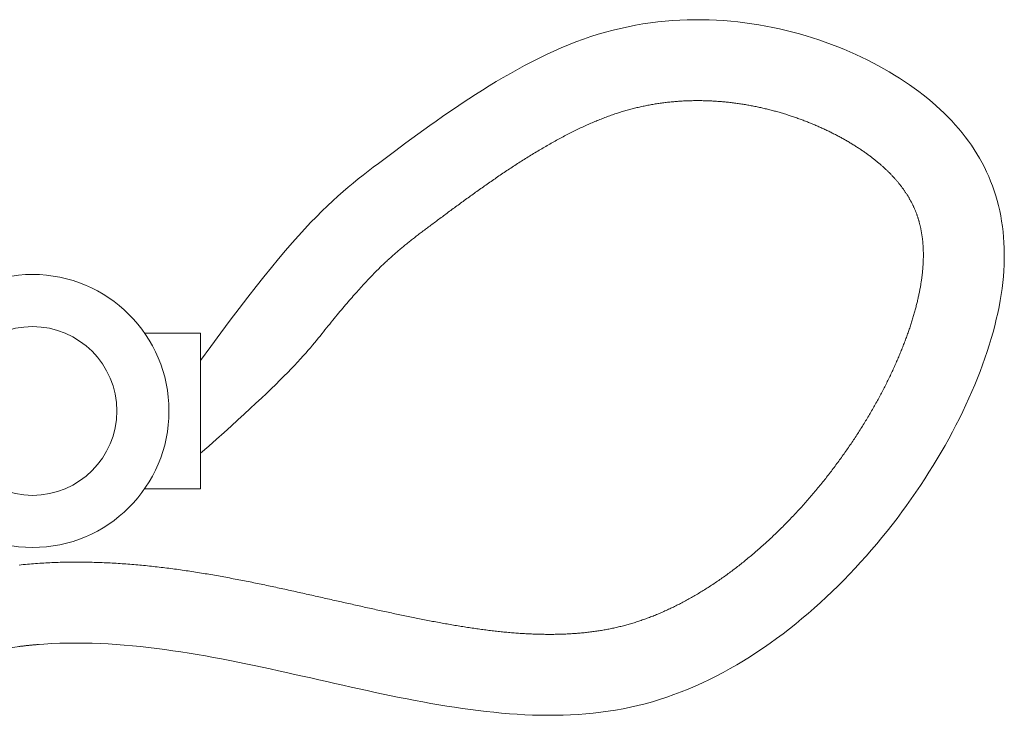
# Model space of a CAD drawing. Units: inches. Extents: x 64 to 1167, y 117 to 939.
# Tile 23 of 56: x 379.191 to 385.274, y 818.434 to 822.731. Entities that reach past the tile are written whole.
import ezdxf

# ---------------------------------------------------------------- set-up
doc = ezdxf.new("R2010")
doc.units = ezdxf.units.IN
doc.header["$MEASUREMENT"] = 0
doc.layers.add('A-FLOR-FIXT', color=8, linetype='Continuous', lineweight=18)

# ---------------------------------------------------------------- blocks, each defined once
blk = doc.blocks.new('FAUCET')
blk.add_lwpolyline([(2.8559, 1.7995), (3.2005, 1.7995), (3.2005, 2.7601), (2.8559, 2.7601)])
for points in [[(3.2005, 2.5912, 0), (3.2645, 2.6791, 0), (3.3257, 2.762, 0), (3.384, 2.8402, 0), (3.4397, 2.9138, 0), (3.493, 2.9831, 0), (3.5438, 3.0482, 0), (3.5924, 3.1094, 0), (3.639, 3.1668, 0), (3.6835, 3.2206, 0), (3.7262, 3.2711, 0), (3.7672, 3.3184, 0), (3.8067, 3.3628, 0), (3.8447, 3.4044, 0), (3.8814, 3.4435, 0), (3.9169, 3.4802, 0), (3.9514, 3.5148, 0), (3.985, 3.5473, 0), (4.0178, 3.5782, 0), (4.05, 3.6075, 0), (4.0816, 3.6354, 0), (4.1129, 3.6621, 0), (4.144, 3.6879, 0), (4.175, 3.713, 0), (4.2059, 3.7375, 0), (4.2371, 3.7616, 0), (4.2685, 3.7856, 0), (4.3004, 3.8096, 0), (4.3329, 3.8338, 0), (4.366, 3.8585, 0), (4.3999, 3.8837, 0), (4.4345, 3.9094, 0), (4.4699, 3.9356, 0), (4.506, 3.9621, 0), (4.5427, 3.989, 0), (4.5802, 4.0161, 0), (4.6182, 4.0434, 0), (4.6569, 4.0709, 0), (4.6961, 4.0984, 0), (4.7359, 4.126, 0), (4.7762, 4.1535, 0), (4.817, 4.181, 0), (4.8584, 4.2082, 0), (4.9002, 4.2353, 0), (4.9424, 4.2621, 0), (4.985, 4.2886, 0), (5.0281, 4.3147, 0), (5.0715, 4.3404, 0), (5.1152, 4.3655, 0), (5.1593, 4.3901, 0), (5.2036, 4.4141, 0), (5.2483, 4.4374, 0), (5.2931, 4.46, 0), (5.3382, 4.4817, 0), (5.3835, 4.5026, 0), (5.429, 4.5226, 0), (5.4746, 4.5416, 0), (5.5203, 4.5596, 0), (5.5662, 4.5765, 0), (5.6121, 4.5923, 0), (5.6581, 4.6068, 0), (5.7041, 4.6202, 0), (5.7502, 4.6325, 0), (5.7962, 4.6436, 0), (5.8423, 4.6537, 0), (5.8883, 4.6626, 0), (5.9343, 4.6705, 0), (5.9802, 4.6773, 0), (6.0261, 4.6831, 0), (6.0718, 4.6878, 0), (6.1175, 4.6916, 0), (6.163, 4.6944, 0), (6.2084, 4.6962, 0), (6.2536, 4.697, 0), (6.2986, 4.697, 0), (6.3435, 4.696, 0), (6.3882, 4.6942, 0), (6.4326, 4.6915, 0), (6.4768, 4.6879, 0), (6.5207, 4.6835, 0), (6.5644, 4.6782, 0), (6.6078, 4.6722, 0), (6.6509, 4.6654, 0), (6.6936, 4.6578, 0), (6.736, 4.6495, 0), (6.7781, 4.6405, 0), (6.8198, 4.6308, 0), (6.8611, 4.6203, 0), (6.902, 4.6092, 0), (6.9425, 4.5975, 0), (6.9825, 4.5851, 0), (7.0221, 4.5721, 0), (7.0612, 4.5585, 0), (7.0999, 4.5443, 0), (7.138, 4.5295, 0), (7.1756, 4.5143, 0), (7.2127, 4.4985, 0), (7.2492, 4.4821, 0), (7.2852, 4.4653, 0), (7.3206, 4.4481, 0), (7.3553, 4.4303, 0), (7.3895, 4.4122, 0), (7.423, 4.3936, 0), (7.4559, 4.3746, 0), (7.4881, 4.3553, 0), (7.5196, 4.3356, 0), (7.5504, 4.3155, 0), (7.5806, 4.2951, 0), (7.61, 4.2744, 0), (7.6387, 4.2533, 0), (7.6666, 4.2319, 0), (7.6939, 4.2101, 0), (7.7205, 4.188, 0), (7.7463, 4.1655, 0), (7.7714, 4.1426, 0), (7.7957, 4.1195, 0), (7.8193, 4.0959, 0), (7.8422, 4.072, 0), (7.8643, 4.0478, 0), (7.8857, 4.0231, 0), (7.9064, 3.9982, 0), (7.9262, 3.9728, 0), (7.9454, 3.9471, 0), (7.9637, 3.921, 0), (7.9813, 3.8946, 0), (7.9981, 3.8678, 0), (8.0142, 3.8406, 0), (8.0294, 3.8131, 0), (8.0439, 3.7852, 0), (8.0576, 3.7569, 0), (8.0705, 3.7282, 0), (8.0827, 3.6991, 0), (8.094, 3.6697, 0), (8.1045, 3.6399, 0), (8.1142, 3.6097, 0), (8.1231, 3.5791, 0), (8.1312, 3.5482, 0), (8.1385, 3.5168, 0), (8.145, 3.4851, 0), (8.1507, 3.453, 0), (8.1555, 3.4204, 0), (8.1595, 3.3875, 0), (8.1626, 3.3542, 0), (8.165, 3.3205, 0), (8.1665, 3.2864, 0), (8.1671, 3.252, 0), (8.1669, 3.2171, 0), (8.1659, 3.1818, 0), (8.164, 3.1461, 0), (8.1612, 3.11, 0), (8.1576, 3.0735, 0), (8.1531, 3.0366, 0), (8.1477, 2.9992, 0), (8.1415, 2.9615, 0), (8.1344, 2.9234, 0), (8.1264, 2.8849, 0), (8.1176, 2.846, 0), (8.108, 2.8068, 0), (8.0975, 2.7673, 0), (8.0862, 2.7275, 0), (8.074, 2.6874, 0), (8.0611, 2.647, 0), (8.0474, 2.6065, 0), (8.0329, 2.5657, 0), (8.0176, 2.5247, 0), (8.0016, 2.4835, 0), (7.9848, 2.4422, 0), (7.9672, 2.4008, 0), (7.9489, 2.3592, 0), (7.9299, 2.3176, 0), (7.9102, 2.2759, 0), (7.8898, 2.2341, 0), (7.8686, 2.1924, 0), (7.8468, 2.1506, 0), (7.8243, 2.1088, 0), (7.8011, 2.0671, 0), (7.7772, 2.0254, 0), (7.7527, 1.9838, 0), (7.7276, 1.9423, 0), (7.7018, 1.9009, 0), (7.6754, 1.8597, 0), (7.6484, 1.8186, 0), (7.6207, 1.7777, 0), (7.5925, 1.737, 0), (7.5637, 1.6965, 0), (7.5343, 1.6563, 0), (7.5043, 1.6163, 0), (7.4738, 1.5766, 0), (7.4428, 1.5372, 0), (7.4112, 1.4981, 0), (7.379, 1.4594, 0), (7.3464, 1.4211, 0), (7.3132, 1.3831, 0), (7.2795, 1.3456, 0), (7.2453, 1.3085, 0), (7.2107, 1.2718, 0), (7.1755, 1.2356, 0), (7.1399, 1.1999, 0), (7.1039, 1.1647, 0), (7.0674, 1.13, 0), (7.0305, 1.0959, 0), (6.9931, 1.0624, 0), (6.9553, 1.0294, 0), (6.9171, 0.9971, 0), (6.8785, 0.9654, 0), (6.8396, 0.9344, 0), (6.8002, 0.904, 0), (6.7605, 0.8744, 0), (6.7204, 0.8455, 0), (6.6799, 0.8173, 0), (6.6391, 0.7898, 0), (6.598, 0.7632, 0), (6.5566, 0.7373, 0), (6.5148, 0.7123, 0), (6.4727, 0.6881, 0), (6.4304, 0.6648, 0), (6.3877, 0.6424, 0), (6.3448, 0.6208, 0), (6.3016, 0.6002, 0), (6.2581, 0.5806, 0), (6.2144, 0.5619, 0), (6.1705, 0.5442, 0), (6.1263, 0.5275, 0), (6.0819, 0.5119, 0), (6.0373, 0.4973, 0), (5.9925, 0.4837, 0), (5.9475, 0.4713, 0), (5.9023, 0.4599, 0), (5.8569, 0.4497, 0), (5.8114, 0.4404, 0), (5.7657, 0.4322, 0), (5.7198, 0.425, 0), (5.6737, 0.4187, 0), (5.6275, 0.4134, 0), (5.5811, 0.409, 0), (5.5345, 0.4055, 0), (5.4878, 0.4029, 0), (5.441, 0.401, 0), (5.394, 0.4, 0), (5.3468, 0.3998, 0), (5.2995, 0.4004, 0), (5.2521, 0.4017, 0), (5.2045, 0.4036, 0), (5.1568, 0.4063, 0), (5.109, 0.4096, 0), (5.0611, 0.4136, 0), (5.013, 0.4182, 0), (4.9648, 0.4233, 0), (4.9165, 0.429, 0), (4.8681, 0.4352, 0), (4.8196, 0.4419, 0), (4.771, 0.4491, 0), (4.7222, 0.4568, 0), (4.6734, 0.4648, 0), (4.6245, 0.4733, 0), (4.5755, 0.4822, 0), (4.5264, 0.4913, 0), (4.4772, 0.5008, 0), (4.428, 0.5106, 0), (4.3786, 0.5207, 0), (4.3292, 0.531, 0), (4.2798, 0.5415, 0), (4.2302, 0.5522, 0), (4.1806, 0.5631, 0), (4.131, 0.5741, 0), (4.0812, 0.5853, 0), (4.0315, 0.5965, 0), (3.9816, 0.6078, 0), (3.9318, 0.6191, 0), (3.8819, 0.6304, 0), (3.8319, 0.6417, 0), (3.7819, 0.6529, 0), (3.7319, 0.6641, 0), (3.6819, 0.6752, 0), (3.6318, 0.6862, 0), (3.5817, 0.697, 0), (3.5316, 0.7077, 0), (3.4815, 0.7182, 0), (3.4313, 0.7284, 0), (3.3812, 0.7384, 0), (3.331, 0.7481, 0), (3.2809, 0.7575, 0), (3.2307, 0.7666, 0), (3.1806, 0.7753, 0), (3.1304, 0.7837, 0), (3.0803, 0.7916, 0), (3.0302, 0.7991, 0), (2.9801, 0.8062, 0), (2.93, 0.8128, 0), (2.88, 0.8188, 0), (2.83, 0.8244, 0), (2.78, 0.8293, 0), (2.73, 0.8337, 0), (2.6801, 0.8375, 0), (2.6302, 0.8406, 0), (2.5804, 0.8431, 0), (2.5307, 0.8449, 0), (2.4809, 0.846, 0), (2.4313, 0.8463, 0), (2.3817, 0.8458, 0), (2.3321, 0.8446, 0), (2.2827, 0.8426, 0), (2.2333, 0.8397, 0), (2.1839, 0.8359, 0), (2.1347, 0.8312, 0), (2.0855, 0.8256, 0), (2.0364, 0.8191, 0)], [(3.2005, 2.0185, 0), (3.2517, 2.0633, 0), (3.3003, 2.1062, 0), (3.3465, 2.1473, 0), (3.3904, 2.1866, 0), (3.4319, 2.2242, 0), (3.4713, 2.2602, 0), (3.5085, 2.2945, 0), (3.5437, 2.3273, 0), (3.5769, 2.3586, 0), (3.6083, 2.3884, 0), (3.6378, 2.4169, 0), (3.6656, 2.444, 0), (3.6917, 2.4699, 0), (3.7163, 2.4945, 0), (3.7394, 2.518, 0), (3.761, 2.5404, 0), (3.7814, 2.5617, 0), (3.8004, 2.582, 0), (3.8183, 2.6014, 0), (3.8351, 2.6199, 0), (3.8509, 2.6376, 0), (3.8657, 2.6545, 0), (3.8797, 2.6707, 0), (3.8929, 2.6862, 0), (3.9054, 2.7011, 0), (3.9172, 2.7154, 0), (3.9286, 2.7293, 0), (3.9394, 2.7427, 0), (3.9499, 2.7557, 0), (3.96, 2.7684, 0), (3.9699, 2.7808, 0), (3.9797, 2.7931, 0), (3.9893, 2.8051, 0), (3.9989, 2.8169, 0), (4.0083, 2.8285, 0), (4.0176, 2.84, 0), (4.0268, 2.8512, 0), (4.0359, 2.8623, 0), (4.0449, 2.8732, 0), (4.0538, 2.8839, 0), (4.0625, 2.8945, 0), (4.0712, 2.9048, 0), (4.0798, 2.9151, 0), (4.0883, 2.9251, 0), (4.0967, 2.935, 0), (4.1049, 2.9447, 0), (4.1131, 2.9542, 0), (4.1212, 2.9636, 0), (4.1292, 2.9729, 0), (4.1371, 2.9819, 0), (4.145, 2.9909, 0), (4.1527, 2.9996, 0), (4.1603, 3.0083, 0), (4.1679, 3.0168, 0), (4.1754, 3.0251, 0), (4.1828, 3.0333, 0), (4.1901, 3.0414, 0), (4.1973, 3.0493, 0), (4.2045, 3.0572, 0), (4.2116, 3.0648, 0), (4.2186, 3.0724, 0), (4.2256, 3.0798, 0), (4.2324, 3.0871, 0), (4.2392, 3.0943, 0), (4.246, 3.1013, 0), (4.2526, 3.1083, 0), (4.2592, 3.1151, 0), (4.2658, 3.1219, 0), (4.2722, 3.1285, 0), (4.2786, 3.135, 0), (4.285, 3.1414, 0), (4.2913, 3.1477, 0), (4.2975, 3.1539, 0), (4.3037, 3.16, 0), (4.3098, 3.166, 0), (4.3159, 3.1719, 0), (4.3219, 3.1777, 0), (4.3279, 3.1835, 0), (4.3338, 3.1891, 0), (4.3397, 3.1947, 0), (4.3456, 3.2002, 0), (4.3514, 3.2057, 0), (4.3572, 3.211, 0), (4.3629, 3.2164, 0), (4.3687, 3.2216, 0), (4.3744, 3.2268, 0), (4.3801, 3.2319, 0), (4.3857, 3.237, 0), (4.3914, 3.242, 0), (4.397, 3.247, 0), (4.4026, 3.252, 0), (4.4082, 3.2569, 0), (4.4138, 3.2617, 0), (4.4194, 3.2665, 0), (4.425, 3.2713, 0), (4.4306, 3.2761, 0), (4.4362, 3.2808, 0), (4.4418, 3.2855, 0), (4.4474, 3.2902, 0), (4.453, 3.2948, 0), (4.4587, 3.2995, 0), (4.4643, 3.3041, 0), (4.47, 3.3087, 0), (4.4756, 3.3133, 0), (4.4813, 3.3179, 0), (4.4871, 3.3224, 0), (4.4928, 3.327, 0), (4.4986, 3.3316, 0), (4.5044, 3.3362, 0), (4.5103, 3.3408, 0), (4.5161, 3.3454, 0), (4.5221, 3.35, 0), (4.528, 3.3546, 0), (4.534, 3.3592, 0), (4.5401, 3.3639, 0), (4.5462, 3.3685, 0), (4.5523, 3.3732, 0), (4.5585, 3.378, 0), (4.5648, 3.3827, 0), (4.5711, 3.3875, 0), (4.5775, 3.3923, 0), (4.5839, 3.3972, 0), (4.5905, 3.4021, 0), (4.597, 3.407, 0), (4.6037, 3.412, 0), (4.6104, 3.417, 0), (4.6172, 3.4221, 0), (4.624, 3.4272, 0), (4.6309, 3.4324, 0), (4.6379, 3.4376, 0), (4.6448, 3.4428, 0), (4.6519, 3.448, 0), (4.659, 3.4533, 0), (4.6661, 3.4586, 0), (4.6733, 3.464, 0), (4.6805, 3.4694, 0), (4.6877, 3.4748, 0), (4.695, 3.4802, 0), (4.7024, 3.4856, 0), (4.7097, 3.4911, 0), (4.7171, 3.4966, 0), (4.7246, 3.5021, 0), (4.732, 3.5076, 0), (4.7395, 3.5132, 0), (4.747, 3.5187, 0), (4.7546, 3.5243, 0), (4.7621, 3.5299, 0), (4.7697, 3.5355, 0), (4.7773, 3.541, 0), (4.7849, 3.5466, 0), (4.7926, 3.5523, 0), (4.8002, 3.5579, 0), (4.8079, 3.5635, 0), (4.8156, 3.5691, 0), (4.8232, 3.5747, 0), (4.8309, 3.5803, 0), (4.8386, 3.5859, 0), (4.8464, 3.5915, 0), (4.8541, 3.5972, 0), (4.8619, 3.6028, 0), (4.8696, 3.6084, 0), (4.8774, 3.614, 0), (4.8852, 3.6196, 0), (4.8931, 3.6253, 0), (4.9009, 3.6309, 0), (4.9088, 3.6365, 0), (4.9167, 3.6421, 0), (4.9246, 3.6478, 0), (4.9325, 3.6534, 0), (4.9404, 3.659, 0), (4.9484, 3.6646, 0), (4.9563, 3.6702, 0), (4.9643, 3.6758, 0), (4.9723, 3.6814, 0), (4.9803, 3.687, 0), (4.9883, 3.6926, 0), (4.9964, 3.6982, 0), (5.0044, 3.7038, 0), (5.0125, 3.7094, 0), (5.0206, 3.7149, 0), (5.0286, 3.7205, 0), (5.0367, 3.726, 0), (5.0449, 3.7316, 0), (5.053, 3.7371, 0), (5.0611, 3.7426, 0), (5.0693, 3.7481, 0), (5.0774, 3.7536, 0), (5.0856, 3.7591, 0), (5.0938, 3.7645, 0), (5.102, 3.77, 0), (5.1102, 3.7754, 0), (5.1184, 3.7808, 0), (5.1266, 3.7862, 0), (5.1349, 3.7916, 0), (5.1431, 3.797, 0), (5.1514, 3.8023, 0), (5.1596, 3.8077, 0), (5.1679, 3.813, 0), (5.1762, 3.8183, 0), (5.1844, 3.8235, 0), (5.1927, 3.8288, 0), (5.201, 3.834, 0), (5.2093, 3.8393, 0), (5.2176, 3.8444, 0), (5.2259, 3.8496, 0), (5.2342, 3.8548, 0), (5.2425, 3.8599, 0), (5.2509, 3.865, 0), (5.2592, 3.8701, 0), (5.2675, 3.8751, 0), (5.2758, 3.8801, 0), (5.2841, 3.8851, 0), (5.2925, 3.8901, 0), (5.3008, 3.8951, 0), (5.3091, 3.9, 0), (5.3174, 3.9049, 0), (5.3258, 3.9097, 0), (5.3341, 3.9146, 0), (5.3424, 3.9194, 0), (5.3507, 3.9241, 0), (5.359, 3.9289, 0), (5.3673, 3.9336, 0), (5.3757, 3.9382, 0), (5.384, 3.9429, 0), (5.3923, 3.9475, 0), (5.4005, 3.9521, 0), (5.4088, 3.9566, 0), (5.4171, 3.9611, 0), (5.4254, 3.9656, 0), (5.4337, 3.97, 0), (5.4419, 3.9744, 0), (5.4502, 3.9788, 0), (5.4584, 3.9831, 0), (5.4667, 3.9874, 0), (5.4749, 3.9916, 0), (5.4831, 3.9959, 0), (5.4913, 4, 0), (5.4995, 4.0042, 0), (5.5077, 4.0082, 0), (5.5159, 4.0123, 0), (5.5241, 4.0163, 0), (5.5322, 4.0203, 0), (5.5403, 4.0242, 0), (5.5485, 4.028, 0), (5.5566, 4.0319, 0), (5.5647, 4.0357, 0), (5.5728, 4.0394, 0), (5.5808, 4.0431, 0), (5.5889, 4.0467, 0), (5.5969, 4.0503, 0), (5.6049, 4.0539, 0), (5.6129, 4.0574, 0), (5.6209, 4.0608, 0), (5.6288, 4.0642, 0), (5.6367, 4.0676, 0), (5.6446, 4.0708, 0), (5.6525, 4.0741, 0), (5.6604, 4.0773, 0), (5.6682, 4.0804, 0), (5.676, 4.0835, 0), (5.6838, 4.0866, 0), (5.6916, 4.0896, 0), (5.6994, 4.0926, 0), (5.7072, 4.0955, 0), (5.7149, 4.0983, 0), (5.7226, 4.1012, 0), (5.7304, 4.1039, 0), (5.7381, 4.1067, 0), (5.7457, 4.1093, 0), (5.7534, 4.112, 0), (5.7611, 4.1146, 0), (5.7687, 4.1171, 0), (5.7764, 4.1196, 0), (5.784, 4.1221, 0), (5.7916, 4.1245, 0), (5.7992, 4.1269, 0), (5.8069, 4.1292, 0), (5.8144, 4.1315, 0), (5.822, 4.1337, 0), (5.8296, 4.1359, 0), (5.8372, 4.1381, 0), (5.8448, 4.1402, 0), (5.8523, 4.1422, 0), (5.8599, 4.1443, 0), (5.8674, 4.1462, 0), (5.875, 4.1482, 0), (5.8825, 4.1501, 0), (5.89, 4.1519, 0), (5.8976, 4.1538, 0), (5.9051, 4.1555, 0), (5.9126, 4.1573, 0), (5.9202, 4.159, 0), (5.9277, 4.1606, 0), (5.9352, 4.1623, 0), (5.9428, 4.1638, 0), (5.9503, 4.1654, 0), (5.9578, 4.1669, 0), (5.9654, 4.1683, 0), (5.9729, 4.1698, 0), (5.9804, 4.1712, 0), (5.988, 4.1725, 0), (5.9955, 4.1738, 0), (6.0031, 4.1751, 0), (6.0106, 4.1763, 0), (6.0182, 4.1775, 0), (6.0257, 4.1787, 0), (6.0333, 4.1798, 0), (6.0409, 4.1809, 0), (6.0485, 4.182, 0), (6.056, 4.183, 0), (6.0636, 4.184, 0), (6.0712, 4.1849, 0), (6.0788, 4.1858, 0), (6.0864, 4.1867, 0), (6.094, 4.1875, 0), (6.1016, 4.1883, 0), (6.1092, 4.1891, 0), (6.1168, 4.1898, 0), (6.1244, 4.1905, 0), (6.132, 4.1912, 0), (6.1396, 4.1918, 0), (6.1472, 4.1924, 0), (6.1548, 4.193, 0), (6.1624, 4.1935, 0), (6.17, 4.194, 0), (6.1776, 4.1944, 0), (6.1852, 4.1948, 0), (6.1928, 4.1952, 0), (6.2004, 4.1956, 0), (6.208, 4.1959, 0), (6.2155, 4.1961, 0), (6.2231, 4.1964, 0), (6.2307, 4.1966, 0), (6.2383, 4.1968, 0), (6.2459, 4.1969, 0), (6.2534, 4.197, 0), (6.261, 4.1971, 0), (6.2686, 4.1971, 0), (6.2761, 4.1971, 0), (6.2837, 4.1971, 0), (6.2913, 4.197, 0), (6.2988, 4.1969, 0), (6.3064, 4.1968, 0), (6.3139, 4.1967, 0), (6.3215, 4.1965, 0), (6.329, 4.1962, 0), (6.3365, 4.196, 0), (6.3441, 4.1957, 0), (6.3516, 4.1954, 0), (6.3591, 4.195, 0), (6.3666, 4.1946, 0), (6.3741, 4.1942, 0), (6.3817, 4.1937, 0), (6.3892, 4.1933, 0), (6.3967, 4.1927, 0), (6.4042, 4.1922, 0), (6.4116, 4.1916, 0), (6.4191, 4.191, 0), (6.4266, 4.1904, 0), (6.4341, 4.1897, 0), (6.4415, 4.189, 0), (6.449, 4.1883, 0), (6.4564, 4.1875, 0), (6.4639, 4.1867, 0), (6.4713, 4.1859, 0), (6.4788, 4.185, 0), (6.4862, 4.1841, 0), (6.4936, 4.1832, 0), (6.501, 4.1823, 0), (6.5084, 4.1813, 0), (6.5158, 4.1803, 0), (6.5232, 4.1793, 0), (6.5306, 4.1782, 0), (6.5379, 4.1771, 0), (6.5453, 4.176, 0), (6.5527, 4.1748, 0), (6.56, 4.1736, 0), (6.5673, 4.1724, 0), (6.5747, 4.1712, 0), (6.582, 4.1699, 0), (6.5893, 4.1686, 0), (6.5966, 4.1673, 0), (6.6039, 4.1659, 0), (6.6112, 4.1645, 0), (6.6185, 4.1631, 0), (6.6257, 4.1616, 0), (6.633, 4.1602, 0), (6.6402, 4.1587, 0), (6.6474, 4.1571, 0), (6.6546, 4.1556, 0), (6.6618, 4.154, 0), (6.669, 4.1524, 0), (6.6762, 4.1507, 0), (6.6834, 4.1491, 0), (6.6905, 4.1474, 0), (6.6977, 4.1457, 0), (6.7048, 4.1439, 0), (6.7119, 4.1421, 0), (6.719, 4.1403, 0), (6.7261, 4.1385, 0), (6.7332, 4.1367, 0), (6.7403, 4.1348, 0), (6.7473, 4.1329, 0), (6.7543, 4.131, 0), (6.7613, 4.129, 0), (6.7683, 4.1271, 0), (6.7753, 4.1251, 0), (6.7823, 4.123, 0), (6.7893, 4.121, 0), (6.7962, 4.1189, 0), (6.8031, 4.1168, 0), (6.81, 4.1147, 0), (6.8169, 4.1126, 0), (6.8238, 4.1104, 0), (6.8307, 4.1082, 0), (6.8375, 4.106, 0), (6.8443, 4.1038, 0), (6.8511, 4.1016, 0), (6.8579, 4.0993, 0), (6.8647, 4.097, 0), (6.8714, 4.0947, 0), (6.8782, 4.0924, 0), (6.8849, 4.09, 0), (6.8916, 4.0876, 0), (6.8982, 4.0852, 0), (6.9049, 4.0828, 0), (6.9115, 4.0804, 0), (6.9181, 4.0779, 0), (6.9247, 4.0754, 0), (6.9313, 4.0729, 0), (6.9379, 4.0704, 0), (6.9444, 4.0679, 0), (6.9509, 4.0653, 0), (6.9574, 4.0628, 0), (6.9639, 4.0602, 0), (6.9703, 4.0576, 0), (6.9767, 4.0549, 0), (6.9831, 4.0523, 0), (6.9895, 4.0496, 0), (6.9959, 4.047, 0), (7.0022, 4.0443, 0), (7.0085, 4.0415, 0), (7.0148, 4.0388, 0), (7.0211, 4.0361, 0), (7.0273, 4.0333, 0), (7.0335, 4.0305, 0), (7.0397, 4.0277, 0), (7.0459, 4.0249, 0), (7.052, 4.0221, 0), (7.0582, 4.0192, 0), (7.0642, 4.0164, 0), (7.0703, 4.0135, 0), (7.0764, 4.0106, 0), (7.0824, 4.0077, 0), (7.0884, 4.0048, 0), (7.0943, 4.0018, 0), (7.1003, 3.9989, 0), (7.1062, 3.9959, 0), (7.1121, 3.9929, 0), (7.1179, 3.99, 0), (7.1238, 3.987, 0), (7.1296, 3.9839, 0), (7.1353, 3.9809, 0), (7.1411, 3.9779, 0), (7.1468, 3.9748, 0), (7.1525, 3.9717, 0), (7.1582, 3.9687, 0), (7.1638, 3.9656, 0), (7.1694, 3.9625, 0), (7.175, 3.9593, 0), (7.1805, 3.9562, 0), (7.186, 3.9531, 0), (7.1915, 3.9499, 0), (7.197, 3.9468, 0), (7.2024, 3.9436, 0), (7.2078, 3.9404, 0), (7.2131, 3.9372, 0), (7.2185, 3.934, 0), (7.2238, 3.9308, 0), (7.229, 3.9276, 0), (7.2343, 3.9244, 0), (7.2395, 3.9211, 0), (7.2447, 3.9179, 0), (7.2498, 3.9146, 0), (7.2549, 3.9114, 0), (7.26, 3.9081, 0), (7.265, 3.9048, 0), (7.27, 3.9015, 0), (7.2749, 3.8983, 0), (7.2798, 3.895, 0), (7.2847, 3.8917, 0), (7.2895, 3.8884, 0), (7.2943, 3.8851, 0), (7.2991, 3.8819, 0), (7.3038, 3.8786, 0), (7.3085, 3.8753, 0), (7.3131, 3.872, 0), (7.3177, 3.8687, 0), (7.3223, 3.8654, 0), (7.3268, 3.8621, 0), (7.3313, 3.8588, 0), (7.3357, 3.8555, 0), (7.3401, 3.8522, 0), (7.3445, 3.8489, 0), (7.3488, 3.8456, 0), (7.3531, 3.8423, 0), (7.3574, 3.839, 0), (7.3616, 3.8357, 0), (7.3658, 3.8324, 0), (7.37, 3.8291, 0), (7.3741, 3.8258, 0), (7.3782, 3.8224, 0), (7.3822, 3.8191, 0), (7.3862, 3.8158, 0), (7.3902, 3.8125, 0), (7.3941, 3.8092, 0), (7.398, 3.8059, 0), (7.4019, 3.8025, 0), (7.4057, 3.7992, 0), (7.4095, 3.7959, 0), (7.4133, 3.7926, 0), (7.417, 3.7892, 0), (7.4207, 3.7859, 0), (7.4243, 3.7826, 0), (7.4279, 3.7793, 0), (7.4315, 3.7759, 0), (7.4351, 3.7726, 0), (7.4386, 3.7693, 0), (7.4421, 3.7659, 0), (7.4455, 3.7626, 0), (7.4489, 3.7593, 0), (7.4523, 3.7559, 0), (7.4557, 3.7526, 0), (7.459, 3.7493, 0), (7.4623, 3.7459, 0), (7.4655, 3.7426, 0), (7.4687, 3.7393, 0), (7.4719, 3.7359, 0), (7.4751, 3.7326, 0), (7.4782, 3.7293, 0), (7.4813, 3.7259, 0), (7.4843, 3.7226, 0), (7.4874, 3.7193, 0), (7.4903, 3.7159, 0), (7.4933, 3.7126, 0), (7.4962, 3.7093, 0), (7.4991, 3.7059, 0), (7.502, 3.7026, 0), (7.5048, 3.6992, 0), (7.5076, 3.6959, 0), (7.5104, 3.6926, 0), (7.5132, 3.6892, 0), (7.5159, 3.6859, 0), (7.5185, 3.6826, 0), (7.5212, 3.6792, 0), (7.5238, 3.6759, 0), (7.5264, 3.6726, 0), (7.529, 3.6692, 0), (7.5315, 3.6659, 0), (7.534, 3.6626, 0), (7.5365, 3.6592, 0), (7.5389, 3.6559, 0), (7.5413, 3.6526, 0), (7.5437, 3.6492, 0), (7.5461, 3.6459, 0), (7.5484, 3.6426, 0), (7.5507, 3.6392, 0), (7.553, 3.6359, 0), (7.5552, 3.6326, 0), (7.5574, 3.6293, 0), (7.5597, 3.6259, 0), (7.5618, 3.6226, 0), (7.564, 3.6193, 0), (7.5661, 3.6159, 0), (7.5682, 3.6126, 0), (7.5703, 3.6092, 0), (7.5724, 3.6059, 0), (7.5744, 3.6026, 0), (7.5764, 3.5992, 0), (7.5784, 3.5959, 0), (7.5803, 3.5925, 0), (7.5823, 3.5891, 0), (7.5842, 3.5858, 0), (7.5861, 3.5824, 0), (7.5879, 3.579, 0), (7.5898, 3.5757, 0), (7.5916, 3.5723, 0), (7.5934, 3.5689, 0), (7.5952, 3.5655, 0), (7.5969, 3.5621, 0), (7.5987, 3.5587, 0), (7.6004, 3.5553, 0), (7.602, 3.5518, 0), (7.6037, 3.5484, 0), (7.6053, 3.545, 0), (7.6069, 3.5415, 0), (7.6085, 3.538, 0), (7.6101, 3.5346, 0), (7.6116, 3.5311, 0), (7.6132, 3.5276, 0), (7.6147, 3.5241, 0), (7.6161, 3.5206, 0), (7.6176, 3.5171, 0), (7.619, 3.5136, 0), (7.6204, 3.51, 0), (7.6218, 3.5065, 0), (7.6232, 3.5029, 0), (7.6245, 3.4994, 0), (7.6259, 3.4958, 0), (7.6272, 3.4922, 0), (7.6284, 3.4886, 0), (7.6297, 3.4849, 0), (7.6309, 3.4813, 0), (7.6322, 3.4777, 0), (7.6333, 3.474, 0), (7.6345, 3.4703, 0), (7.6357, 3.4666, 0), (7.6368, 3.4629, 0), (7.6379, 3.4592, 0), (7.639, 3.4555, 0), (7.6401, 3.4517, 0), (7.6411, 3.4479, 0), (7.6421, 3.4441, 0), (7.6432, 3.4403, 0), (7.6441, 3.4365, 0), (7.6451, 3.4327, 0), (7.646, 3.4288, 0), (7.647, 3.4249, 0), (7.6479, 3.4211, 0), (7.6488, 3.4171, 0), (7.6496, 3.4132, 0), (7.6505, 3.4093, 0), (7.6513, 3.4053, 0), (7.6521, 3.4013, 0), (7.6529, 3.3973, 0), (7.6536, 3.3933, 0), (7.6544, 3.3892, 0), (7.6551, 3.3852, 0), (7.6558, 3.3811, 0), (7.6565, 3.377, 0), (7.6572, 3.3728, 0), (7.6578, 3.3687, 0), (7.6584, 3.3645, 0), (7.6591, 3.3603, 0), (7.6596, 3.3561, 0), (7.6602, 3.3518, 0), (7.6608, 3.3475, 0), (7.6613, 3.3432, 0), (7.6618, 3.3389, 0), (7.6623, 3.3346, 0), (7.6628, 3.3302, 0), (7.6632, 3.3258, 0), (7.6636, 3.3213, 0), (7.664, 3.3169, 0), (7.6644, 3.3124, 0), (7.6647, 3.3079, 0), (7.6651, 3.3033, 0), (7.6654, 3.2988, 0), (7.6657, 3.2941, 0), (7.6659, 3.2895, 0), (7.6661, 3.2849, 0), (7.6663, 3.2802, 0), (7.6665, 3.2755, 0), (7.6667, 3.2707, 0), (7.6668, 3.2659, 0), (7.6669, 3.2611, 0), (7.667, 3.2563, 0), (7.6671, 3.2514, 0), (7.6671, 3.2466, 0), (7.6671, 3.2416, 0), (7.6671, 3.2367, 0), (7.667, 3.2317, 0), (7.6669, 3.2267, 0), (7.6668, 3.2217, 0), (7.6667, 3.2166, 0), (7.6666, 3.2115, 0), (7.6664, 3.2064, 0), (7.6662, 3.2012, 0), (7.6659, 3.1961, 0), (7.6657, 3.1908, 0), (7.6654, 3.1856, 0), (7.665, 3.1803, 0), (7.6647, 3.175, 0), (7.6643, 3.1697, 0), (7.6639, 3.1643, 0), (7.6635, 3.1589, 0), (7.663, 3.1535, 0), (7.6625, 3.148, 0), (7.662, 3.1426, 0), (7.6614, 3.137, 0), (7.6608, 3.1315, 0), (7.6602, 3.1259, 0), (7.6596, 3.1203, 0), (7.6589, 3.1147, 0), (7.6582, 3.109, 0), (7.6574, 3.1033, 0), (7.6567, 3.0975, 0), (7.6559, 3.0918, 0), (7.655, 3.086, 0), (7.6542, 3.0801, 0), (7.6533, 3.0743, 0), (7.6524, 3.0684, 0), (7.6514, 3.0625, 0), (7.6504, 3.0565, 0), (7.6494, 3.0505, 0), (7.6483, 3.0445, 0), (7.6472, 3.0384, 0), (7.6461, 3.0324, 0), (7.645, 3.0262, 0), (7.6438, 3.0201, 0), (7.6425, 3.0139, 0), (7.6413, 3.0077, 0), (7.64, 3.0014, 0), (7.6387, 2.9951, 0), (7.6373, 2.9888, 0), (7.6359, 2.9825, 0), (7.6345, 2.9761, 0), (7.633, 2.9697, 0), (7.6315, 2.9632, 0), (7.63, 2.9567, 0), (7.6284, 2.9502, 0), (7.6268, 2.9437, 0), (7.6252, 2.9371, 0), (7.6235, 2.9305, 0), (7.6218, 2.9238, 0), (7.62, 2.9171, 0), (7.6182, 2.9104, 0), (7.6164, 2.9037, 0), (7.6146, 2.8969, 0), (7.6127, 2.8901, 0), (7.6107, 2.8832, 0), (7.6088, 2.8764, 0), (7.6067, 2.8695, 0), (7.6047, 2.8626, 0), (7.6026, 2.8556, 0), (7.6005, 2.8487, 0), (7.5984, 2.8417, 0), (7.5962, 2.8347, 0), (7.594, 2.8277, 0), (7.5917, 2.8206, 0), (7.5894, 2.8135, 0), (7.5871, 2.8064, 0), (7.5848, 2.7993, 0), (7.5824, 2.7921, 0), (7.58, 2.785, 0), (7.5775, 2.7778, 0), (7.575, 2.7706, 0), (7.5725, 2.7634, 0), (7.5699, 2.7561, 0), (7.5673, 2.7488, 0), (7.5647, 2.7415, 0), (7.562, 2.7342, 0), (7.5593, 2.7269, 0), (7.5566, 2.7196, 0), (7.5538, 2.7122, 0), (7.551, 2.7048, 0), (7.5482, 2.6974, 0), (7.5453, 2.69, 0), (7.5424, 2.6826, 0), (7.5395, 2.6751, 0), (7.5365, 2.6677, 0), (7.5335, 2.6602, 0), (7.5305, 2.6527, 0), (7.5274, 2.6452, 0), (7.5243, 2.6376, 0), (7.5212, 2.6301, 0), (7.518, 2.6225, 0), (7.5148, 2.615, 0), (7.5116, 2.6074, 0), (7.5083, 2.5998, 0), (7.505, 2.5922, 0), (7.5017, 2.5846, 0), (7.4984, 2.5769, 0), (7.495, 2.5693, 0), (7.4915, 2.5616, 0), (7.4881, 2.554, 0), (7.4846, 2.5463, 0), (7.4811, 2.5386, 0), (7.4775, 2.5309, 0), (7.4739, 2.5232, 0), (7.4703, 2.5155, 0), (7.4667, 2.5077, 0), (7.463, 2.5, 0), (7.4593, 2.4923, 0), (7.4555, 2.4845, 0), (7.4518, 2.4767, 0), (7.448, 2.469, 0), (7.4441, 2.4612, 0), (7.4403, 2.4534, 0), (7.4364, 2.4456, 0), (7.4324, 2.4378, 0), (7.4285, 2.43, 0), (7.4245, 2.4222, 0), (7.4205, 2.4144, 0), (7.4164, 2.4066, 0), (7.4123, 2.3987, 0), (7.4082, 2.3909, 0), (7.4041, 2.3831, 0), (7.3999, 2.3753, 0), (7.3957, 2.3674, 0), (7.3915, 2.3596, 0), (7.3872, 2.3517, 0), (7.3829, 2.3439, 0), (7.3786, 2.336, 0), (7.3742, 2.3282, 0), (7.3699, 2.3203, 0), (7.3654, 2.3125, 0), (7.361, 2.3046, 0), (7.3565, 2.2968, 0), (7.352, 2.2889, 0), (7.3475, 2.2811, 0), (7.3429, 2.2732, 0), (7.3383, 2.2653, 0), (7.3337, 2.2575, 0), (7.3291, 2.2496, 0), (7.3244, 2.2418, 0), (7.3197, 2.2339, 0), (7.315, 2.2261, 0), (7.3102, 2.2182, 0), (7.3054, 2.2104, 0), (7.3006, 2.2026, 0), (7.2958, 2.1947, 0), (7.2909, 2.1869, 0), (7.286, 2.1791, 0), (7.2811, 2.1712, 0), (7.2762, 2.1634, 0), (7.2712, 2.1556, 0), (7.2662, 2.1478, 0), (7.2612, 2.1399, 0), (7.2561, 2.1321, 0), (7.251, 2.1243, 0), (7.2459, 2.1165, 0), (7.2408, 2.1087, 0), (7.2356, 2.1009, 0), (7.2304, 2.0932, 0), (7.2252, 2.0854, 0), (7.22, 2.0776, 0), (7.2147, 2.0699, 0), (7.2094, 2.0621, 0), (7.2041, 2.0543, 0), (7.1988, 2.0466, 0), (7.1934, 2.0389, 0), (7.188, 2.0311, 0), (7.1826, 2.0234, 0), (7.1772, 2.0157, 0), (7.1717, 2.008, 0), (7.1662, 2.0003, 0), (7.1607, 1.9926, 0), (7.1552, 1.985, 0), (7.1496, 1.9773, 0), (7.144, 1.9697, 0), (7.1384, 1.962, 0), (7.1328, 1.9544, 0), (7.1272, 1.9468, 0), (7.1215, 1.9391, 0), (7.1158, 1.9316, 0), (7.1101, 1.924, 0), (7.1043, 1.9164, 0), (7.0986, 1.9088, 0), (7.0928, 1.9013, 0), (7.087, 1.8937, 0), (7.0811, 1.8862, 0), (7.0753, 1.8787, 0), (7.0694, 1.8712, 0), (7.0635, 1.8637, 0), (7.0576, 1.8562, 0), (7.0516, 1.8488, 0), (7.0457, 1.8413, 0), (7.0397, 1.8339, 0), (7.0337, 1.8265, 0), (7.0276, 1.8191, 0), (7.0216, 1.8117, 0), (7.0155, 1.8043, 0), (7.0094, 1.797, 0), (7.0033, 1.7896, 0), (6.9972, 1.7823, 0), (6.991, 1.775, 0), (6.9849, 1.7677, 0), (6.9787, 1.7604, 0), (6.9725, 1.7532, 0), (6.9662, 1.746, 0), (6.96, 1.7387, 0), (6.9537, 1.7315, 0), (6.9474, 1.7244, 0), (6.9411, 1.7172, 0), (6.9348, 1.71, 0), (6.9284, 1.7029, 0), (6.9221, 1.6958, 0), (6.9157, 1.6887, 0), (6.9093, 1.6817, 0), (6.9029, 1.6746, 0), (6.8964, 1.6676, 0), (6.89, 1.6606, 0), (6.8835, 1.6536, 0), (6.877, 1.6466, 0), (6.8705, 1.6397, 0), (6.864, 1.6328, 0), (6.8574, 1.6259, 0), (6.8509, 1.619, 0), (6.8443, 1.6121, 0), (6.8377, 1.6053, 0), (6.8311, 1.5985, 0), (6.8244, 1.5917, 0), (6.8178, 1.5849, 0), (6.8111, 1.5782, 0), (6.8045, 1.5715, 0), (6.7978, 1.5648, 0), (6.7911, 1.5581, 0), (6.7843, 1.5515, 0), (6.7776, 1.5448, 0), (6.7708, 1.5382, 0), (6.7641, 1.5317, 0), (6.7573, 1.5251, 0), (6.7505, 1.5186, 0), (6.7437, 1.5121, 0), (6.7368, 1.5056, 0), (6.73, 1.4992, 0), (6.7231, 1.4927, 0), (6.7163, 1.4864, 0), (6.7094, 1.48, 0), (6.7025, 1.4736, 0), (6.6956, 1.4673, 0), (6.6887, 1.461, 0), (6.6817, 1.4548, 0), (6.6748, 1.4485, 0), (6.6678, 1.4423, 0), (6.6608, 1.4361, 0), (6.6539, 1.43, 0), (6.6469, 1.4238, 0), (6.6398, 1.4177, 0), (6.6328, 1.4117, 0), (6.6258, 1.4056, 0), (6.6187, 1.3996, 0), (6.6117, 1.3936, 0), (6.6046, 1.3877, 0), (6.5975, 1.3818, 0), (6.5905, 1.3759, 0), (6.5834, 1.37, 0), (6.5763, 1.3642, 0), (6.5691, 1.3584, 0), (6.562, 1.3526, 0), (6.5549, 1.3468, 0), (6.5477, 1.3411, 0), (6.5406, 1.3354, 0), (6.5334, 1.3298, 0), (6.5262, 1.3242, 0), (6.519, 1.3186, 0), (6.5118, 1.313, 0), (6.5046, 1.3075, 0), (6.4974, 1.302, 0), (6.4902, 1.2965, 0), (6.483, 1.2911, 0), (6.4757, 1.2857, 0), (6.4685, 1.2803, 0), (6.4612, 1.275, 0), (6.454, 1.2697, 0), (6.4467, 1.2645, 0), (6.4394, 1.2592, 0), (6.4322, 1.254, 0), (6.4249, 1.2489, 0), (6.4176, 1.2438, 0), (6.4103, 1.2387, 0), (6.403, 1.2336, 0), (6.3956, 1.2286, 0), (6.3883, 1.2236, 0), (6.381, 1.2187, 0), (6.3737, 1.2137, 0), (6.3663, 1.2089, 0), (6.359, 1.204, 0), (6.3517, 1.1992, 0), (6.3443, 1.1944, 0), (6.3369, 1.1897, 0), (6.3296, 1.185, 0), (6.3222, 1.1804, 0), (6.3149, 1.1757, 0), (6.3075, 1.1711, 0), (6.3001, 1.1666, 0), (6.2927, 1.1621, 0), (6.2854, 1.1576, 0), (6.278, 1.1532, 0), (6.2706, 1.1488, 0), (6.2632, 1.1444, 0), (6.2558, 1.1401, 0), (6.2484, 1.1358, 0), (6.241, 1.1315, 0), (6.2336, 1.1273, 0), (6.2262, 1.1232, 0), (6.2188, 1.119, 0), (6.2114, 1.1149, 0), (6.204, 1.1109, 0), (6.1966, 1.1068, 0), (6.1892, 1.1029, 0), (6.1818, 1.0989, 0), (6.1744, 1.095, 0), (6.167, 1.0911, 0), (6.1595, 1.0873, 0), (6.1521, 1.0835, 0), (6.1447, 1.0798, 0), (6.1373, 1.0761, 0), (6.1299, 1.0724, 0), (6.1225, 1.0688, 0), (6.1151, 1.0652, 0), (6.1077, 1.0616, 0), (6.1003, 1.0581, 0), (6.0929, 1.0546, 0), (6.0855, 1.0512, 0), (6.0781, 1.0478, 0), (6.0707, 1.0445, 0), (6.0633, 1.0411, 0), (6.0559, 1.0379, 0), (6.0485, 1.0346, 0), (6.0411, 1.0314, 0), (6.0337, 1.0283, 0), (6.0263, 1.0252, 0), (6.0189, 1.0221, 0), (6.0115, 1.0191, 0), (6.0042, 1.0161, 0), (5.9968, 1.0132, 0), (5.9894, 1.0103, 0), (5.982, 1.0074, 0), (5.9747, 1.0046, 0), (5.9673, 1.0018, 0), (5.96, 0.9991, 0), (5.9526, 0.9964, 0), (5.9453, 0.9937, 0), (5.9379, 0.9911, 0), (5.9306, 0.9886, 0), (5.9233, 0.986, 0), (5.9159, 0.9835, 0), (5.9086, 0.9811, 0), (5.9013, 0.9787, 0), (5.894, 0.9763, 0), (5.8866, 0.974, 0), (5.8793, 0.9717, 0), (5.872, 0.9695, 0), (5.8646, 0.9673, 0), (5.8573, 0.9651, 0), (5.85, 0.963, 0), (5.8427, 0.9609, 0), (5.8353, 0.9589, 0), (5.828, 0.9569, 0), (5.8206, 0.9549, 0), (5.8133, 0.953, 0), (5.8059, 0.9511, 0), (5.7985, 0.9493, 0), (5.7912, 0.9475, 0), (5.7838, 0.9457, 0), (5.7764, 0.9439, 0), (5.769, 0.9422, 0), (5.7616, 0.9406, 0), (5.7541, 0.939, 0), (5.7467, 0.9374, 0), (5.7392, 0.9358, 0), (5.7318, 0.9343, 0), (5.7243, 0.9328, 0), (5.7168, 0.9314, 0), (5.7093, 0.9299, 0), (5.7018, 0.9286, 0), (5.6942, 0.9272, 0), (5.6867, 0.9259, 0), (5.6791, 0.9246, 0), (5.6715, 0.9234, 0), (5.6639, 0.9222, 0), (5.6563, 0.921, 0), (5.6486, 0.9199, 0), (5.6409, 0.9188, 0), (5.6333, 0.9177, 0), (5.6255, 0.9166, 0), (5.6178, 0.9156, 0), (5.61, 0.9146, 0), (5.6023, 0.9137, 0), (5.5944, 0.9128, 0), (5.5866, 0.9119, 0), (5.5787, 0.911, 0), (5.5709, 0.9102, 0), (5.5629, 0.9094, 0), (5.555, 0.9087, 0), (5.547, 0.9079, 0), (5.5391, 0.9072, 0), (5.531, 0.9066, 0), (5.523, 0.9059, 0), (5.515, 0.9053, 0), (5.5069, 0.9048, 0), (5.4988, 0.9042, 0), (5.4907, 0.9037, 0), (5.4825, 0.9033, 0), (5.4744, 0.9028, 0), (5.4662, 0.9024, 0), (5.458, 0.902, 0), (5.4498, 0.9017, 0), (5.4415, 0.9014, 0), (5.4333, 0.9011, 0), (5.425, 0.9008, 0), (5.4167, 0.9006, 0), (5.4083, 0.9004, 0), (5.4, 0.9002, 0), (5.3916, 0.9001, 0), (5.3832, 0.9, 0), (5.3748, 0.8999, 0), (5.3663, 0.8999, 0), (5.3579, 0.8998, 0), (5.3494, 0.8999, 0), (5.3409, 0.8999, 0), (5.3324, 0.9, 0), (5.3238, 0.9001, 0), (5.3152, 0.9002, 0), (5.3067, 0.9004, 0), (5.298, 0.9005, 0), (5.2894, 0.9008, 0), (5.2808, 0.901, 0), (5.2721, 0.9013, 0), (5.2634, 0.9016, 0), (5.2547, 0.9019, 0), (5.2459, 0.9023, 0), (5.2372, 0.9027, 0), (5.2284, 0.9031, 0), (5.2196, 0.9035, 0), (5.2107, 0.904, 0), (5.2019, 0.9045, 0), (5.193, 0.905, 0), (5.1841, 0.9056, 0), (5.1752, 0.9062, 0), (5.1663, 0.9068, 0), (5.1573, 0.9074, 0), (5.1484, 0.9081, 0), (5.1394, 0.9088, 0), (5.1303, 0.9095, 0), (5.1213, 0.9103, 0), (5.1122, 0.911, 0), (5.1032, 0.9118, 0), (5.0941, 0.9127, 0), (5.0849, 0.9135, 0), (5.0758, 0.9144, 0), (5.0666, 0.9153, 0), (5.0575, 0.9163, 0), (5.0483, 0.9172, 0), (5.039, 0.9182, 0), (5.0298, 0.9192, 0), (5.0205, 0.9203, 0), (5.0113, 0.9213, 0), (5.002, 0.9224, 0), (4.9927, 0.9235, 0), (4.9833, 0.9247, 0), (4.974, 0.9258, 0), (4.9646, 0.927, 0), (4.9552, 0.9282, 0), (4.9458, 0.9295, 0), (4.9364, 0.9307, 0), (4.9269, 0.932, 0), (4.9174, 0.9333, 0), (4.908, 0.9347, 0), (4.8984, 0.936, 0), (4.8889, 0.9374, 0), (4.8794, 0.9388, 0), (4.8698, 0.9402, 0), (4.8602, 0.9417, 0), (4.8506, 0.9431, 0), (4.841, 0.9446, 0), (4.8314, 0.9461, 0), (4.8217, 0.9476, 0), (4.8121, 0.9492, 0), (4.8024, 0.9507, 0), (4.7927, 0.9523, 0), (4.783, 0.9539, 0), (4.7732, 0.9556, 0), (4.7635, 0.9572, 0), (4.7537, 0.9589, 0), (4.7439, 0.9606, 0), (4.7341, 0.9623, 0), (4.7243, 0.964, 0), (4.7144, 0.9657, 0), (4.7045, 0.9675, 0), (4.6947, 0.9693, 0), (4.6848, 0.9711, 0), (4.6749, 0.9729, 0), (4.6649, 0.9747, 0), (4.655, 0.9765, 0), (4.645, 0.9784, 0), (4.635, 0.9803, 0), (4.625, 0.9822, 0), (4.615, 0.9841, 0), (4.605, 0.986, 0), (4.5949, 0.988, 0), (4.5849, 0.9899, 0), (4.5748, 0.9919, 0), (4.5647, 0.9939, 0), (4.5546, 0.9959, 0), (4.5444, 0.9979, 0), (4.5343, 0.9999, 0), (4.5241, 1.002, 0), (4.514, 1.004, 0), (4.5038, 1.0061, 0), (4.4936, 1.0082, 0), (4.4833, 1.0103, 0), (4.4731, 1.0124, 0), (4.4628, 1.0145, 0), (4.4526, 1.0167, 0), (4.4423, 1.0188, 0), (4.432, 1.021, 0), (4.4217, 1.0231, 0), (4.4113, 1.0253, 0), (4.401, 1.0275, 0), (4.3906, 1.0297, 0), (4.3802, 1.032, 0), (4.3698, 1.0342, 0), (4.3594, 1.0364, 0), (4.349, 1.0387, 0), (4.3386, 1.0409, 0), (4.3281, 1.0432, 0), (4.3177, 1.0455, 0), (4.3072, 1.0478, 0), (4.2967, 1.05, 0), (4.2862, 1.0524, 0), (4.2756, 1.0547, 0), (4.2651, 1.057, 0), (4.2546, 1.0593, 0), (4.244, 1.0616, 0), (4.2334, 1.064, 0), (4.2228, 1.0663, 0), (4.2122, 1.0687, 0), (4.2016, 1.0711, 0), (4.1909, 1.0734, 0), (4.1803, 1.0758, 0), (4.1696, 1.0782, 0), (4.1589, 1.0806, 0), (4.1482, 1.083, 0), (4.1375, 1.0854, 0), (4.1268, 1.0878, 0), (4.1161, 1.0902, 0), (4.1053, 1.0926, 0), (4.0946, 1.0951, 0), (4.0838, 1.0975, 0), (4.073, 1.0999, 0), (4.0622, 1.1023, 0), (4.0514, 1.1048, 0), (4.0406, 1.1072, 0), (4.0298, 1.1097, 0), (4.0189, 1.1121, 0), (4.0081, 1.1146, 0), (3.9972, 1.117, 0), (3.9863, 1.1195, 0), (3.9754, 1.1219, 0), (3.9645, 1.1244, 0), (3.9536, 1.1269, 0), (3.9426, 1.1293, 0), (3.9317, 1.1318, 0), (3.9207, 1.1342, 0), (3.9097, 1.1367, 0), (3.8988, 1.1392, 0), (3.8878, 1.1416, 0), (3.8767, 1.1441, 0), (3.8657, 1.1466, 0), (3.8547, 1.149, 0), (3.8437, 1.1515, 0), (3.8326, 1.154, 0), (3.8215, 1.1564, 0), (3.8104, 1.1589, 0), (3.7994, 1.1614, 0), (3.7883, 1.1638, 0), (3.7771, 1.1663, 0), (3.766, 1.1687, 0), (3.7549, 1.1712, 0), (3.7437, 1.1736, 0), (3.7325, 1.1761, 0), (3.7214, 1.1785, 0), (3.7102, 1.1809, 0), (3.699, 1.1834, 0), (3.6878, 1.1858, 0), (3.6765, 1.1882, 0), (3.6653, 1.1906, 0), (3.654, 1.193, 0), (3.6428, 1.1954, 0), (3.6315, 1.1978, 0), (3.6202, 1.2002, 0), (3.6089, 1.2026, 0), (3.5976, 1.205, 0), (3.5863, 1.2073, 0), (3.5749, 1.2097, 0), (3.5636, 1.212, 0), (3.5522, 1.2144, 0), (3.5409, 1.2167, 0), (3.5295, 1.219, 0), (3.5181, 1.2213, 0), (3.5067, 1.2236, 0), (3.4953, 1.2259, 0), (3.4838, 1.2282, 0), (3.4724, 1.2304, 0), (3.4609, 1.2327, 0), (3.4495, 1.2349, 0), (3.438, 1.2371, 0), (3.4265, 1.2394, 0), (3.415, 1.2416, 0), (3.4035, 1.2438, 0), (3.392, 1.2459, 0), (3.3804, 1.2481, 0), (3.3689, 1.2502, 0), (3.3573, 1.2524, 0), (3.3457, 1.2545, 0), (3.3342, 1.2566, 0), (3.3226, 1.2587, 0), (3.311, 1.2607, 0), (3.2993, 1.2628, 0), (3.2877, 1.2648, 0), (3.2761, 1.2669, 0), (3.2644, 1.2689, 0), (3.2527, 1.2708, 0), (3.2411, 1.2728, 0), (3.2294, 1.2748, 0), (3.2177, 1.2767, 0), (3.206, 1.2786, 0), (3.1942, 1.2805, 0), (3.1825, 1.2824, 0), (3.1708, 1.2842, 0), (3.159, 1.2861, 0), (3.1472, 1.2879, 0), (3.1354, 1.2897, 0), (3.1236, 1.2914, 0), (3.1118, 1.2932, 0), (3.1, 1.2949, 0), (3.0882, 1.2966, 0), (3.0764, 1.2983, 0), (3.0645, 1.2999, 0), (3.0526, 1.3016, 0), (3.0408, 1.3032, 0), (3.0289, 1.3048, 0), (3.017, 1.3063, 0), (3.0051, 1.3079, 0), (2.9932, 1.3094, 0), (2.9812, 1.3109, 0), (2.9693, 1.3123, 0), (2.9573, 1.3138, 0), (2.9454, 1.3152, 0), (2.9334, 1.3166, 0), (2.9214, 1.3179, 0), (2.9094, 1.3193, 0), (2.8974, 1.3206, 0), (2.8854, 1.3218, 0), (2.8733, 1.3231, 0), (2.8613, 1.3243, 0), (2.8492, 1.3255, 0), (2.8372, 1.3266, 0), (2.8251, 1.3278, 0), (2.813, 1.3289, 0), (2.8009, 1.3299, 0), (2.7888, 1.331, 0), (2.7767, 1.332, 0), (2.7645, 1.333, 0), (2.7524, 1.3339, 0), (2.7402, 1.3348, 0), (2.7281, 1.3357, 0), (2.7159, 1.3365, 0), (2.7037, 1.3374, 0), (2.6915, 1.3381, 0), (2.6793, 1.3389, 0), (2.6671, 1.3396, 0), (2.6548, 1.3403, 0), (2.6426, 1.3409, 0), (2.6303, 1.3415, 0), (2.6181, 1.3421, 0), (2.6058, 1.3427, 0), (2.5935, 1.3432, 0), (2.5812, 1.3436, 0), (2.5689, 1.3441, 0), (2.5566, 1.3445, 0), (2.5442, 1.3448, 0), (2.5319, 1.3451, 0), (2.5195, 1.3454, 0), (2.5072, 1.3457, 0), (2.4948, 1.3459, 0), (2.4824, 1.346, 0), (2.47, 1.3462, 0), (2.4576, 1.3462, 0), (2.4452, 1.3463, 0), (2.4328, 1.3463, 0), (2.4203, 1.3463, 0), (2.4079, 1.3462, 0), (2.3954, 1.3461, 0), (2.3829, 1.3459, 0), (2.3704, 1.3457, 0), (2.3579, 1.3455, 0), (2.3454, 1.3452, 0), (2.3329, 1.3449, 0), (2.3204, 1.3445, 0), (2.3079, 1.3441, 0), (2.2953, 1.3436, 0), (2.2828, 1.3431, 0), (2.2702, 1.3425, 0), (2.2576, 1.3419, 0), (2.2451, 1.3413, 0), (2.2325, 1.3406, 0), (2.2199, 1.3398, 0), (2.2073, 1.339, 0), (2.1946, 1.3382, 0), (2.182, 1.3373, 0), (2.1694, 1.3363, 0), (2.1567, 1.3354, 0), (2.1441, 1.3343, 0), (2.1314, 1.3332, 0), (2.1188, 1.3321, 0), (2.1061, 1.3309, 0), (2.0934, 1.3296, 0), (2.0807, 1.3283, 0)], [(2.2006, 0.8373, 0), (2.1956, 0.8369, 0), (2.1905, 0.8364, 0), (2.1854, 0.836, 0), (2.1804, 0.8356, 0), (2.1753, 0.8351, 0), (2.1702, 0.8347, 0), (2.1652, 0.8342, 0), (2.1601, 0.8337, 0), (2.155, 0.8333, 0), (2.15, 0.8328, 0), (2.1449, 0.8323, 0), (2.1399, 0.8318, 0), (2.1348, 0.8312, 0), (2.1298, 0.8307, 0), (2.1247, 0.8302, 0), (2.1196, 0.8296, 0), (2.1146, 0.8291, 0), (2.1095, 0.8285, 0), (2.1045, 0.8279, 0), (2.0994, 0.8273, 0), (2.0944, 0.8267, 0), (2.0893, 0.8261, 0), (2.0843, 0.8255, 0), (2.0792, 0.8249, 0)], [(2.2006, 0.8373, 0), (2.1956, 0.8369, 0), (2.1905, 0.8364, 0), (2.1854, 0.836, 0), (2.1804, 0.8356, 0), (2.1753, 0.8351, 0), (2.1702, 0.8347, 0), (2.1652, 0.8342, 0), (2.1601, 0.8337, 0), (2.155, 0.8333, 0), (2.15, 0.8328, 0), (2.1449, 0.8323, 0), (2.1399, 0.8318, 0), (2.1348, 0.8312, 0), (2.1298, 0.8307, 0), (2.1247, 0.8302, 0), (2.1196, 0.8296, 0), (2.1146, 0.8291, 0), (2.1095, 0.8285, 0), (2.1045, 0.8279, 0), (2.0994, 0.8273, 0), (2.0944, 0.8267, 0), (2.0893, 0.8261, 0), (2.0843, 0.8255, 0), (2.0792, 0.8249, 0)]]:
    blk.add_polyline3d(points)
for radius in [0.8433, 0.5212]:
    blk.add_circle((2.1627, 2.2798), radius)

msp = doc.modelspace()

# ---------------------------------------------------------------- block references
at = {"layer": 'A-FLOR-FIXT'}
msp.add_blockref('FAUCET', (377.107, 818.034), dxfattribs=at)

doc.saveas('drawing.dxf')
